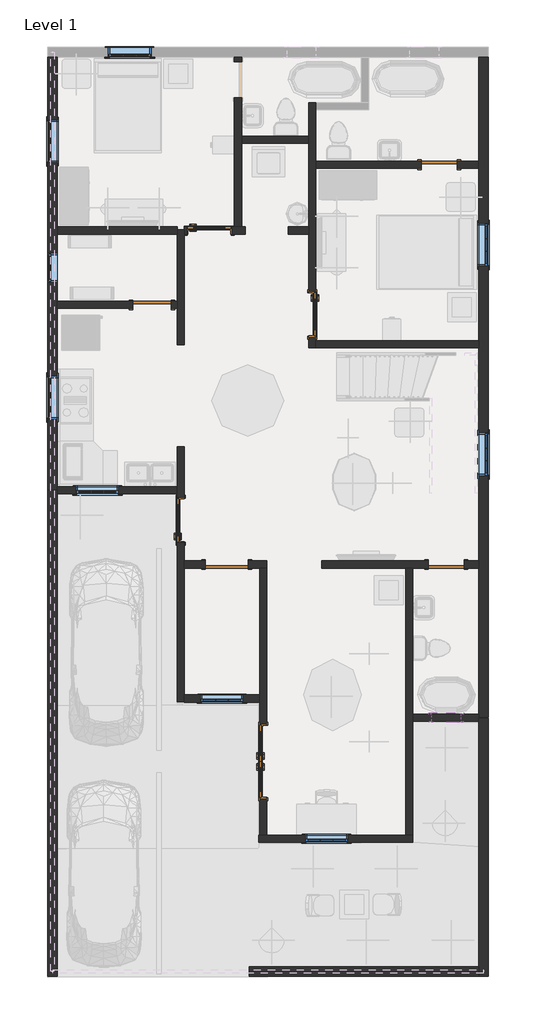
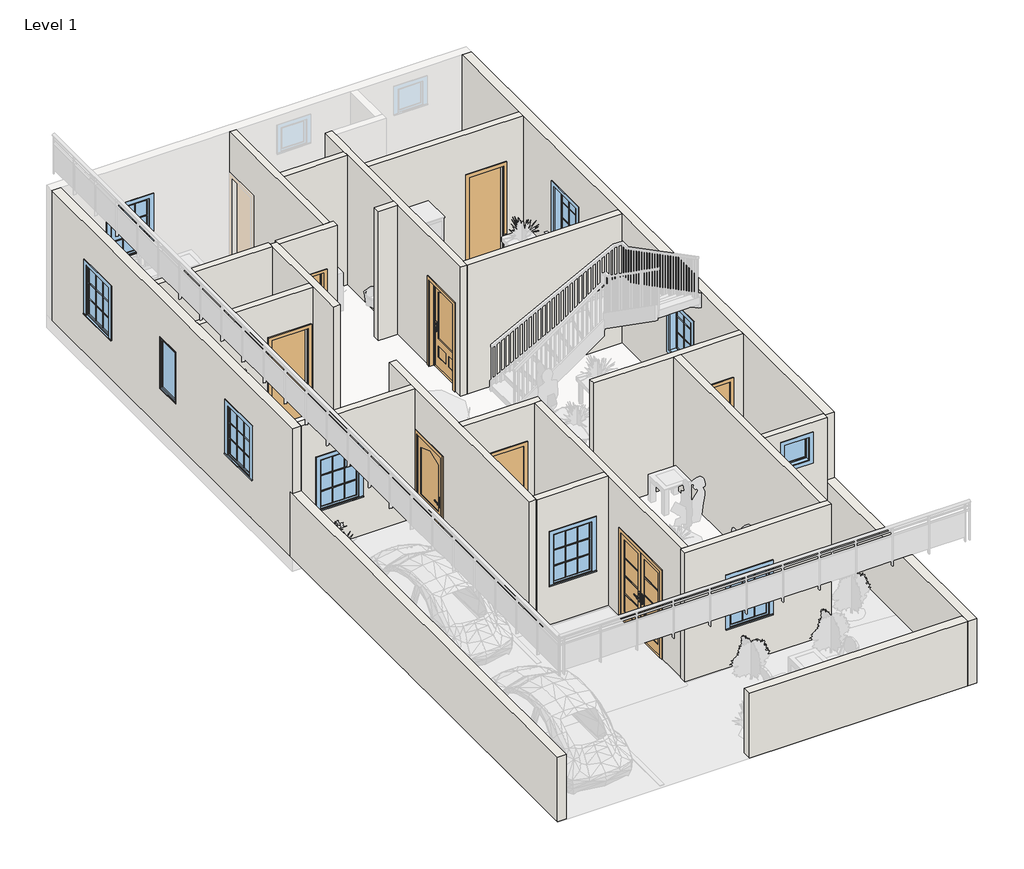
# One storey, part 1 of 4: 24 walls, 10 windows, 8 doors.
"""IFC4 building model written with IfcOpenShell, lengths in millimetres."""

from ifc_helpers import new_model, si_unit, frame, origin, origin_with_axes, place, context, project, spatial, polyline, outline, extrude, faceted_brep, transform, mapped, element, save
from components import door_5d363d20, door_94998e6c, door_255cab33, door_059fdd7e, door_377e7377, door_686f89d2, window_ce5e1bf6, window_29c06734, window_5c190c7e, window_80bd9af0, window_3d781103

model = new_model("IFC4")

# Units and contexts
model_context = context("Model", 3, world=origin())
ifc_project = project(units=[si_unit("LENGTHUNIT", "METRE", prefix="MILLI")], contexts=[model_context])

# Site, building, storey
site = spatial("IfcSite", under=ifc_project)
building = spatial("IfcBuilding", under=site)
storey = spatial("IfcBuildingStorey", under=building, Name="Level 1", Elevation=0.0)

# Doors
placement = place(None, origin())
door_shape = door_5d363d20(model_context)
element("IfcDoor", 1, ObjectType="36\" x 80\"", at=placement, inside=storey, context=model_context, shape_type="MappedRepresentation", body=[
    mapped(door_shape, transform((-8373.0976606, 9970.2021763, 0.0), x_axis=(-1.0, 0.0, 0.0), y_axis=(0.0, -1.0, 0.0), z_axis=(0.0, 0.0, 1.0))),
])
element("IfcDoor", 2, ObjectType="36\" x 80\"", at=placement, inside=storey, context=model_context, shape_type="MappedRepresentation", body=[
    mapped(door_shape, transform((-6185.5226606, 8189.0271763, 0.0), x_axis=(0.0, 1.0, 0.0), y_axis=(-1.0, 0.0, 0.0), z_axis=(0.0, 0.0, 1.0))),
])
element("IfcDoor", 3, ObjectType="36\" x 80\"", at=placement, inside=storey, context=model_context, shape_type="MappedRepresentation", body=[
    mapped(door_shape, transform((-8985.8726606, 3820.2271763, 0.0), x_axis=(0.0, -1.0, 0.0), y_axis=(1.0, 0.0, 0.0), z_axis=(0.0, 0.0, 1.0))),
])
door_2_shape = door_94998e6c(model_context)
element("IfcDoor", 4, ObjectType="Door-Exterior-Double-Full Glass-Wood_Clad : 60\" x 80\"", at=placement, inside=storey, context=model_context, shape_type="MappedRepresentation", body=[
    mapped(door_2_shape, transform((-7233.2726606, -1297.8728237, 0.0), x_axis=(0.0, 1.0, 0.0), y_axis=(-1.0, 0.0, 0.0), z_axis=(0.0, 0.0, 1.0))),
])
door_3_shape = door_255cab33(model_context)
element("IfcDoor", 5, ObjectType="Single-Flush : 30\" x 80\"", at=placement, inside=storey, context=model_context, shape_type="MappedRepresentation", body=[
    mapped(door_3_shape, transform((-3343.8976606, 2880.4271763, 0.0), x_axis=(1.0, 0.0, 0.0), y_axis=(0.0, 1.0, 0.0), z_axis=(0.0, 0.0, 1.0))),
])
door_4_shape = door_059fdd7e(model_context)
element("IfcDoor", 6, ObjectType="Single-Flush : 30\" x 80\"", at=placement, inside=storey, context=model_context, shape_type="MappedRepresentation", body=[
    mapped(door_4_shape, transform((-3496.2976606, 11364.0271763, 0.0), x_axis=(1.0, 0.0, 0.0), y_axis=(0.0, 1.0, 0.0), z_axis=(0.0, 0.0, 1.0))),
])
door_5_shape = door_377e7377(model_context)
element("IfcDoor", 7, ObjectType="Single-Flush : 32\" x 84\"", at=placement, inside=storey, context=model_context, shape_type="MappedRepresentation", body=[
    mapped(door_5_shape, transform((-9592.2976606, 8392.2271763, 0.0), x_axis=(1.0, 0.0, 0.0), y_axis=(0.0, 1.0, 0.0), z_axis=(0.0, 0.0, 1.0))),
])
door_6_shape = door_686f89d2(model_context)
element("IfcDoor", 8, ObjectType="Single-Flush : 36\" x 84\"", at=placement, inside=storey, context=model_context, shape_type="MappedRepresentation", body=[
    mapped(door_6_shape, transform((-8004.7976606, 2880.4271763, 0.0), x_axis=(1.0, 0.0, 0.0), y_axis=(0.0, 1.0, 0.0), z_axis=(0.0, 0.0, 1.0))),
])

# Walls
element("IfcWall", 9, ObjectType="Generic - 5'", at=placement, inside=storey, context=model_context, shape_type="Brep", body=[
    faceted_brep([(-11598.8976606, -5857.1728237, 0.0), (-11598.8976606, 4379.0271763, 0.0), (-11598.8976606, 4455.2271763, 0.0), (-11598.8976606, 4455.2271763, 1524.0), (-11598.8976606, -5857.1728237, 1524.0), (-11802.0976606, -5857.1728237, 0.0), (-11802.0976606, -5857.1728237, 1524.0), (-11802.0976606, 4455.2271763, 1524.0), (-11802.0976606, 4455.2271763, 0.0)], [[[0, 1, 2, 3, 4]], [[5, 6, 7, 8]], [[2, 1, 0, 5, 8]], [[3, 2, 8, 7]], [[4, 3, 7, 6]], [[0, 4, 6, 5]]]),
])
element("IfcWall", 10, ObjectType="Generic - 5'", at=placement, inside=storey, context=model_context, shape_type="Brep", body=[
    faceted_brep([(-2658.0976606, -383.4728237, 0.0), (-2658.0976606, -446.9728237, 0.0), (-2658.0976606, -5653.9728237, 0.0), (-2658.0976606, -5857.1728237, 0.0), (-2658.0976606, -5857.1728237, 1524.0), (-2658.0976606, -5653.9728237, 1524.0), (-2658.0976606, -383.4728237, 1524.0), (-2454.8976606, -383.4728237, 0.0), (-2454.8976606, -383.4728237, 1524.0), (-2454.8976606, -5857.1728237, 1524.0), (-2454.8976606, -5857.1728237, 0.0)], [[[0, 1, 2, 3, 4, 5, 6]], [[7, 8, 9, 10]], [[3, 2, 1, 0, 7, 10]], [[6, 5, 4, 9, 8]], [[0, 6, 8, 7]], [[4, 3, 10, 9]]]),
])
element("IfcWall", 11, ObjectType="Generic - 5'", at=placement, inside=storey, context=model_context, shape_type="SweptSolid", body=[
    extrude(outline(polyline([(-7522.1976606, -5653.9728237), (-2658.0976606, -5653.9728237), (-2658.0976606, -5857.1728237), (-7522.1976606, -5857.1728237), (-7522.1976606, -5653.9728237)])), origin_with_axes(), (0.0, 0.0, 1.0), 1524.0),
])
element("IfcWall", 12, ObjectType="Generic - 8\"", at=placement, inside=storey, context=model_context, shape_type="Brep", body=[
    faceted_brep([(-2658.0976606, 13650.0271763, 0.0), (-2658.0976606, 11440.2271763, 0.0), (-2658.0976606, 11287.8271763, 0.0), (-2658.0976606, 7630.2271763, 0.0), (-2658.0976606, 7477.8271763, 0.0), (-2658.0976606, 2956.6271763, 0.0), (-2658.0976606, 2804.2271763, 0.0), (-2658.0976606, -358.0728237, 0.0), (-2658.0976606, -358.0728237, 3048.0), (-2658.0976606, 2804.2271763, 3048.0), (-2658.0976606, 2956.6271763, 3048.0), (-2658.0976606, 7477.8271763, 3048.0), (-2658.0976606, 7630.2271763, 3048.0), (-2658.0976606, 11287.8271763, 3048.0), (-2658.0976606, 11440.2271763, 3048.0), (-2658.0976606, 13650.0271763, 3048.0), (-2658.0976606, 9205.0271763, 2133.6), (-2658.0976606, 9205.0271763, 914.4), (-2658.0976606, 10119.4271763, 914.4), (-2658.0976606, 10119.4271763, 2133.6), (-2658.0976606, 4760.0271763, 2133.6), (-2658.0976606, 4760.0271763, 914.4), (-2658.0976606, 5674.4271763, 914.4), (-2658.0976606, 5674.4271763, 2133.6), (-2454.8976606, 13650.0271763, 0.0), (-2454.8976606, 13650.0271763, 3048.0), (-2454.8976606, -358.0728237, 3048.0), (-2454.8976606, -358.0728237, 0.0), (-2454.8976606, 9205.0271763, 2133.6), (-2454.8976606, 10119.4271763, 2133.6), (-2454.8976606, 10119.4271763, 914.4), (-2454.8976606, 9205.0271763, 914.4), (-2454.8976606, 4760.0271763, 2133.6), (-2454.8976606, 5674.4271763, 2133.6), (-2454.8976606, 5674.4271763, 914.4), (-2454.8976606, 4760.0271763, 914.4)], [[[0, 1, 2, 3, 4, 5, 6, 7, 8, 9, 10, 11, 12, 13, 14, 15], [16, 17, 18, 19], [20, 21, 22, 23]], [[24, 25, 26, 27], [28, 29, 30, 31], [32, 33, 34, 35]], [[7, 6, 5, 4, 3, 2, 1, 0, 24, 27]], [[8, 7, 27, 26]], [[0, 15, 25, 24]], [[17, 16, 28, 31]], [[18, 17, 31, 30]], [[19, 18, 30, 29]], [[16, 19, 29, 28]], [[21, 20, 32, 35]], [[22, 21, 35, 34]], [[23, 22, 34, 33]], [[20, 23, 33, 32]], [[15, 14, 13, 12, 11, 10, 9, 8, 26, 25]]]),
])
element("IfcWall", 13, ObjectType="Generic - 8\"", at=placement, inside=storey, context=model_context, shape_type="Brep", body=[
    faceted_brep([(-11598.8976606, 4455.2271763, 0.0), (-11598.8976606, 4531.4271763, 0.0), (-11598.8976606, 8316.0271763, 0.0), (-11598.8976606, 8468.4271763, 0.0), (-11598.8976606, 9890.8271763, 0.0), (-11598.8976606, 10043.2271763, 0.0), (-11598.8976606, 13650.0271763, 0.0), (-11598.8976606, 13650.0271763, 3048.0), (-11598.8976606, 10043.2271763, 3048.0), (-11598.8976606, 9890.8271763, 3048.0), (-11598.8976606, 8468.4271763, 3048.0), (-11598.8976606, 8316.0271763, 3048.0), (-11598.8976606, 4531.4271763, 3048.0), (-11598.8976606, 4379.0271763, 3048.0), (-11598.8976606, 4379.0271763, 1524.0), (-11598.8976606, 4455.2271763, 1524.0), (-11598.8976606, 12316.5271763, 2133.6), (-11598.8976606, 12316.5271763, 914.4), (-11598.8976606, 11402.1271763, 914.4), (-11598.8976606, 11402.1271763, 2133.6), (-11598.8976606, 6880.9271763, 2133.6), (-11598.8976606, 6880.9271763, 914.4), (-11598.8976606, 5966.5271763, 914.4), (-11598.8976606, 5966.5271763, 2133.6), (-11598.8976606, 9484.4271763, 2133.6), (-11598.8976606, 9484.4271763, 914.4), (-11598.8976606, 8874.8271763, 914.4), (-11598.8976606, 8874.8271763, 2133.6), (-11802.0976606, 4455.2271763, 0.0), (-11802.0976606, 4455.2271763, 1524.0), (-11802.0976606, 4379.0271763, 1524.0), (-11802.0976606, 4379.0271763, 3048.0), (-11802.0976606, 13650.0271763, 3048.0), (-11802.0976606, 13650.0271763, 0.0), (-11802.0976606, 12316.5271763, 2133.6), (-11802.0976606, 11402.1271763, 2133.6), (-11802.0976606, 11402.1271763, 914.4), (-11802.0976606, 12316.5271763, 914.4), (-11802.0976606, 6880.9271763, 2133.6), (-11802.0976606, 5966.5271763, 2133.6), (-11802.0976606, 5966.5271763, 914.4), (-11802.0976606, 6880.9271763, 914.4), (-11802.0976606, 9484.4271763, 2133.6), (-11802.0976606, 8874.8271763, 2133.6), (-11802.0976606, 8874.8271763, 914.4), (-11802.0976606, 9484.4271763, 914.4)], [[[0, 1, 2, 3, 4, 5, 6, 7, 8, 9, 10, 11, 12, 13, 14, 15], [16, 17, 18, 19], [20, 21, 22, 23], [24, 25, 26, 27]], [[28, 29, 30, 31, 32, 33], [34, 35, 36, 37], [38, 39, 40, 41], [42, 43, 44, 45]], [[6, 5, 4, 3, 2, 1, 0, 28, 33]], [[7, 6, 33, 32]], [[16, 19, 35, 34]], [[19, 18, 36, 35]], [[18, 17, 37, 36]], [[17, 16, 34, 37]], [[20, 23, 39, 38]], [[23, 22, 40, 39]], [[22, 21, 41, 40]], [[21, 20, 38, 41]], [[24, 27, 43, 42]], [[27, 26, 44, 43]], [[26, 25, 45, 44]], [[25, 24, 42, 45]], [[0, 15, 29, 28]], [[14, 30, 29, 15]], [[14, 13, 31, 30]], [[13, 12, 11, 10, 9, 8, 7, 32, 31]]]),
])
element("IfcWall", 14, ObjectType="inner 6\"", at=placement, inside=storey, context=model_context, shape_type="Brep", body=[
    faceted_brep([(-9058.8976606, 10043.2271763, 0.0), (-11598.8976606, 10043.2271763, 0.0), (-11598.8976606, 10043.2271763, 3048.0), (-9058.8976606, 10043.2271763, 3048.0), (-9058.8976606, 9890.8271763, 0.0), (-9058.8976606, 9890.8271763, 3048.0), (-11598.8976606, 9890.8271763, 3048.0), (-11598.8976606, 9890.8271763, 0.0), (-9058.8976606, 9979.7271763, 0.0), (-9058.8976606, 9979.7271763, 3048.0)], [[[0, 1, 2, 3]], [[4, 5, 6, 7]], [[1, 0, 8, 4, 7]], [[0, 3, 9, 5, 4, 8]], [[2, 1, 7, 6]], [[3, 2, 6, 5, 9]]]),
])
element("IfcWall", 15, ObjectType="inner 6\"", at=placement, inside=storey, context=model_context, shape_type="SweptSolid", body=[
    extrude(outline(polyline([(-6264.8976606, 11821.2271763), (-7687.2976606, 11821.2271763), (-7687.2976606, 11973.6271763), (-6264.8976606, 11973.6271763), (-6264.8976606, 11821.2271763)])), origin_with_axes(), (0.0, 0.0, 1.0), 3048.0),
])
element("IfcWall", 16, ObjectType="inner 6\"", at=placement, inside=storey, context=model_context, shape_type="Brep", body=[
    faceted_brep([(-6112.4976606, 12684.8271763, 0.0), (-6112.4976606, 12684.8271763, 3048.0), (-6112.4976606, 12532.4271763, 3048.0), (-6112.4976606, 11440.2271763, 3048.0), (-6112.4976606, 11287.8271763, 3048.0), (-6112.4976606, 7630.2271763, 3048.0), (-6112.4976606, 7477.8271763, 3048.0), (-6112.4976606, 7477.8271763, 0.0), (-6112.4976606, 7630.2271763, 0.0), (-6112.4976606, 7706.4271763, 0.0), (-6112.4976606, 7706.4271763, 2057.4), (-6112.4976606, 8671.6271763, 2057.4), (-6112.4976606, 8671.6271763, 0.0), (-6112.4976606, 11287.8271763, 0.0), (-6112.4976606, 11440.2271763, 0.0), (-6112.4976606, 12532.4271763, 0.0), (-6264.8976606, 12684.8271763, 3048.0), (-6264.8976606, 12684.8271763, 0.0), (-6264.8976606, 11973.6271763, 0.0), (-6264.8976606, 11821.2271763, 0.0), (-6264.8976606, 10043.2271763, 0.0), (-6264.8976606, 9890.8271763, 0.0), (-6264.8976606, 8671.6271763, 0.0), (-6264.8976606, 8671.6271763, 2057.4), (-6264.8976606, 7706.4271763, 2057.4), (-6264.8976606, 7706.4271763, 0.0), (-6264.8976606, 7477.8271763, 0.0), (-6264.8976606, 7477.8271763, 3048.0), (-6264.8976606, 9890.8271763, 3048.0), (-6264.8976606, 10043.2271763, 3048.0), (-6264.8976606, 11821.2271763, 3048.0), (-6264.8976606, 11973.6271763, 3048.0)], [[[0, 1, 2, 3, 4, 5, 6, 7, 8, 9, 10, 11, 12, 13, 14, 15]], [[16, 17, 18, 19, 20, 21, 22, 23, 24, 25, 26, 27, 28, 29, 30, 31]], [[17, 0, 15, 14, 13, 12, 22, 21, 20, 19, 18]], [[7, 26, 25, 9, 8]], [[1, 0, 17, 16]], [[7, 6, 27, 26]], [[11, 23, 22, 12]], [[23, 11, 10, 24]], [[24, 10, 9, 25]], [[6, 5, 4, 3, 2, 1, 16, 31, 30, 29, 28, 27]]]),
])
element("IfcWall", 17, ObjectType="inner 6\"", at=placement, inside=storey, context=model_context, shape_type="SweptSolid", body=[
    extrude(outline(polyline([(-6112.4976606, 7630.2271763), (-2658.0976606, 7630.2271763), (-2658.0976606, 7477.8271763), (-6112.4976606, 7477.8271763), (-6112.4976606, 7630.2271763)])), origin_with_axes(), (0.0, 0.0, 1.0), 3048.0),
])
element("IfcWall", 18, ObjectType="inner 6\"", at=placement, inside=storey, context=model_context, shape_type="SweptSolid", body=[
    extrude(outline(polyline([(2032.0, -3115.2976606), (0.0, -3115.2976606), (0.0, -2658.0976606), (3048.0, -2658.0976606), (3048.0, -6112.4976606), (0.0, -6112.4976606), (0.0, -3877.2976606), (2032.0, -3877.2976606), (2032.0, -3115.2976606)])), frame((0.0, 11287.8271763, 0.0), z_axis=(0.0, 1.0, 0.0), x_axis=(0.0, 0.0, 1.0)), (0.0, 0.0, 1.0), 152.4),
])
element("IfcWall", 19, ObjectType="inner 6\"", at=placement, inside=storey, context=model_context, shape_type="SweptSolid", body=[
    extrude(outline(polyline([(2133.6, -9185.8976606), (0.0, -9185.8976606), (0.0, -9058.8976606), (3048.0, -9058.8976606), (3048.0, -11598.8976606), (0.0, -11598.8976606), (0.0, -9998.6976606), (2133.6, -9998.6976606), (2133.6, -9185.8976606)])), frame((0.0, 8316.0271763, 0.0), z_axis=(0.0, 1.0, 0.0), x_axis=(0.0, 0.0, 1.0)), (0.0, 0.0, 1.0), 152.4),
])
element("IfcWall", 20, ObjectType="inner 6\"", at=placement, inside=storey, context=model_context, shape_type="Brep", body=[
    faceted_brep([(-11598.8976606, 4379.0271763, 3048.0), (-11598.8976606, 4379.0271763, 1524.0), (-11598.8976606, 4379.0271763, 0.0), (-9058.8976606, 4379.0271763, 0.0), (-9058.8976606, 4379.0271763, 3048.0), (-11205.1976606, 4379.0271763, 2133.6), (-10290.7976606, 4379.0271763, 2133.6), (-10290.7976606, 4379.0271763, 914.4), (-11205.1976606, 4379.0271763, 914.4), (-11598.8976606, 4531.4271763, 0.0), (-11598.8976606, 4531.4271763, 3048.0), (-9058.8976606, 4531.4271763, 3048.0), (-9058.8976606, 4531.4271763, 0.0), (-11205.1976606, 4531.4271763, 2133.6), (-11205.1976606, 4531.4271763, 914.4), (-10290.7976606, 4531.4271763, 914.4), (-10290.7976606, 4531.4271763, 2133.6), (-11598.8976606, 4455.2271763, 0.0)], [[[0, 1, 2, 3, 4], [5, 6, 7, 8]], [[9, 10, 11, 12], [13, 14, 15, 16]], [[3, 2, 17, 9, 12]], [[4, 3, 12, 11]], [[14, 13, 5, 8]], [[15, 14, 8, 7]], [[16, 15, 7, 6]], [[13, 16, 6, 5]], [[0, 10, 9, 17, 2, 1]], [[0, 4, 11, 10]]]),
])
element("IfcWall", 21, ObjectType="inner 6\"", at=placement, inside=storey, context=model_context, shape_type="Brep", body=[
    faceted_brep([(-4055.0976606, -2859.9728237, 0.0), (-4055.0976606, -446.9728237, 0.0), (-4055.0976606, -294.5728237, 0.0), (-4055.0976606, 2804.2271763, 0.0), (-4055.0976606, 2804.2271763, 3048.0), (-4055.0976606, -294.5728237, 3048.0), (-4055.0976606, -446.9728237, 3048.0), (-4055.0976606, -2859.9728237, 3048.0), (-4207.4976606, -2859.9728237, 0.0), (-4207.4976606, -2859.9728237, 3048.0), (-4207.4976606, 2804.2271763, 3048.0), (-4207.4976606, 2804.2271763, 0.0)], [[[0, 1, 2, 3, 4, 5, 6, 7]], [[8, 9, 10, 11]], [[3, 2, 1, 0, 8, 11]], [[0, 7, 9, 8]], [[4, 3, 11, 10]], [[7, 6, 5, 4, 10, 9]]]),
])
element("IfcWall", 22, ObjectType="inner 6\"", at=placement, inside=storey, context=model_context, shape_type="Brep", body=[
    faceted_brep([(-4055.0976606, -446.9728237, 0.0), (-2658.0976606, -446.9728237, 0.0), (-2658.0976606, -446.9728237, 3048.0), (-4055.0976606, -446.9728237, 3048.0), (-3039.0976606, -446.9728237, 2768.6), (-3039.0976606, -446.9728237, 2159.0), (-3648.6976606, -446.9728237, 2159.0), (-3648.6976606, -446.9728237, 2768.6), (-4055.0976606, -294.5728237, 0.0), (-4055.0976606, -294.5728237, 3048.0), (-2658.0976606, -294.5728237, 3048.0), (-2658.0976606, -294.5728237, 0.0), (-3039.0976606, -294.5728237, 2768.6), (-3648.6976606, -294.5728237, 2768.6), (-3648.6976606, -294.5728237, 2159.0), (-3039.0976606, -294.5728237, 2159.0), (-2658.0976606, -383.4728237, 0.0)], [[[0, 1, 2, 3], [4, 5, 6, 7]], [[8, 9, 10, 11], [12, 13, 14, 15]], [[1, 0, 8, 11, 16]], [[0, 3, 9, 8]], [[2, 1, 16, 11, 10]], [[5, 4, 12, 15]], [[6, 5, 15, 14]], [[7, 6, 14, 13]], [[4, 7, 13, 12]], [[3, 2, 10, 9]]]),
])
element("IfcWall", 23, ObjectType="inner 6\"", at=placement, inside=storey, context=model_context, shape_type="Brep", body=[
    faceted_brep([(-2962.8976606, 2804.2271763, 2032.0), (-2962.8976606, 2804.2271763, 0.0), (-2658.0976606, 2804.2271763, 0.0), (-2658.0976606, 2804.2271763, 3048.0), (-4055.0976606, 2804.2271763, 3048.0), (-4207.4976606, 2804.2271763, 3048.0), (-5985.4976606, 2804.2271763, 3048.0), (-5985.4976606, 2804.2271763, 0.0), (-4207.4976606, 2804.2271763, 0.0), (-4055.0976606, 2804.2271763, 0.0), (-3724.8976606, 2804.2271763, 0.0), (-3724.8976606, 2804.2271763, 2032.0), (-2658.0976606, 2956.6271763, 0.0), (-2962.8976606, 2956.6271763, 0.0), (-2962.8976606, 2956.6271763, 2032.0), (-3724.8976606, 2956.6271763, 2032.0), (-3724.8976606, 2956.6271763, 0.0), (-5985.4976606, 2956.6271763, 0.0), (-5985.4976606, 2956.6271763, 3048.0), (-2658.0976606, 2956.6271763, 3048.0)], [[[0, 1, 2, 3, 4, 5, 6, 7, 8, 9, 10, 11]], [[12, 13, 14, 15, 16, 17, 18, 19]], [[2, 1, 13, 12]], [[10, 9, 8, 7, 17, 16]], [[7, 6, 18, 17]], [[3, 2, 12, 19]], [[14, 13, 1, 0]], [[15, 14, 0, 11]], [[16, 15, 11, 10]], [[6, 5, 4, 3, 19, 18]]]),
])
element("IfcWall", 24, ObjectType="inner 6\"", at=placement, inside=storey, context=model_context, shape_type="Brep", body=[
    faceted_brep([(-7153.8976606, 2956.6271763, 0.0), (-7547.5976606, 2956.6271763, 0.0), (-7547.5976606, 2956.6271763, 2133.6), (-8461.9976606, 2956.6271763, 2133.6), (-8461.9976606, 2956.6271763, 0.0), (-8906.4976606, 2956.6271763, 0.0), (-8906.4976606, 2956.6271763, 3048.0), (-7153.8976606, 2956.6271763, 3048.0), (-7547.5976606, 2804.2271763, 2133.6), (-7547.5976606, 2804.2271763, 0.0), (-7306.2976606, 2804.2271763, 0.0), (-7153.8976606, 2804.2271763, 0.0), (-7153.8976606, 2804.2271763, 3048.0), (-7306.2976606, 2804.2271763, 3048.0), (-8906.4976606, 2804.2271763, 3048.0), (-8906.4976606, 2804.2271763, 0.0), (-8461.9976606, 2804.2271763, 0.0), (-8461.9976606, 2804.2271763, 2133.6)], [[[0, 1, 2, 3, 4, 5, 6, 7]], [[8, 9, 10, 11, 12, 13, 14, 15, 16, 17]], [[16, 15, 5, 4]], [[11, 10, 9, 1, 0]], [[0, 7, 12, 11]], [[6, 5, 15, 14]], [[2, 1, 9, 8]], [[3, 2, 8, 17]], [[4, 3, 17, 16]], [[7, 6, 14, 13, 12]]]),
])
element("IfcWall", 25, ObjectType="inner 6\"", at=placement, inside=storey, context=model_context, shape_type="Brep", body=[
    faceted_brep([(-7306.2976606, -2859.9728237, 0.0), (-7306.2976606, -2859.9728237, 3048.0), (-7306.2976606, -40.5728237, 3048.0), (-7306.2976606, 111.8271763, 3048.0), (-7306.2976606, 2804.2271763, 3048.0), (-7306.2976606, 2804.2271763, 0.0), (-7306.2976606, 111.8271763, 0.0), (-7306.2976606, -40.5728237, 0.0), (-7306.2976606, -510.4728237, 0.0), (-7306.2976606, -510.4728237, 2057.4), (-7306.2976606, -2085.2728237, 2057.4), (-7306.2976606, -2085.2728237, 0.0), (-7153.8976606, -2859.9728237, 3048.0), (-7153.8976606, -2859.9728237, 0.0), (-7153.8976606, -2085.2728237, 0.0), (-7153.8976606, -2085.2728237, 2057.4), (-7153.8976606, -510.4728237, 2057.4), (-7153.8976606, -510.4728237, 0.0), (-7153.8976606, 2804.2271763, 0.0), (-7153.8976606, 2804.2271763, 3048.0)], [[[0, 1, 2, 3, 4, 5, 6, 7, 8, 9, 10, 11]], [[12, 13, 14, 15, 16, 17, 18, 19]], [[13, 0, 11, 14]], [[5, 18, 17, 8, 7, 6]], [[1, 0, 13, 12]], [[5, 4, 19, 18]], [[16, 9, 8, 17]], [[9, 16, 15, 10]], [[10, 15, 14, 11]], [[4, 3, 2, 1, 12, 19]]]),
])
element("IfcWall", 26, ObjectType="inner 6\"", at=placement, inside=storey, context=model_context, shape_type="Brep", body=[
    faceted_brep([(-9058.8976606, 9979.7271763, 0.0), (-9058.8976606, 9890.8271763, 0.0), (-9058.8976606, 8468.4271763, 0.0), (-9058.8976606, 8316.0271763, 0.0), (-9058.8976606, 7541.3271763, 0.0), (-9058.8976606, 7541.3271763, 3048.0), (-9058.8976606, 8316.0271763, 3048.0), (-9058.8976606, 8468.4271763, 3048.0), (-9058.8976606, 9890.8271763, 3048.0), (-9058.8976606, 9979.7271763, 3048.0), (-8906.4976606, 9979.7271763, 0.0), (-8906.4976606, 9979.7271763, 3048.0), (-8906.4976606, 9890.8271763, 3048.0), (-8906.4976606, 7541.3271763, 3048.0), (-8906.4976606, 7541.3271763, 0.0), (-8906.4976606, 9890.8271763, 0.0)], [[[0, 1, 2, 3, 4, 5, 6, 7, 8, 9]], [[10, 11, 12, 13, 14, 15]], [[4, 3, 2, 1, 0, 10, 15, 14]], [[5, 4, 14, 13]], [[0, 9, 11, 10]], [[9, 8, 7, 6, 5, 13, 12, 11]]]),
])
element("IfcWall", 27, ObjectType="inner 6\"", at=placement, inside=storey, context=model_context, shape_type="Brep", body=[
    faceted_brep([(-7839.6976606, 13650.0271763, 0.0), (-7839.6976606, 13548.4271763, 0.0), (-7839.6976606, 13548.4271763, 2032.0), (-7839.6976606, 12786.4271763, 2032.0), (-7839.6976606, 12786.4271763, 0.0), (-7839.6976606, 10043.2271763, 0.0), (-7839.6976606, 10043.2271763, 3048.0), (-7839.6976606, 13650.0271763, 3048.0), (-7687.2976606, 13548.4271763, 2032.0), (-7687.2976606, 13548.4271763, 0.0), (-7687.2976606, 13650.0271763, 0.0), (-7687.2976606, 13650.0271763, 3048.0), (-7687.2976606, 11973.6271763, 3048.0), (-7687.2976606, 11821.2271763, 3048.0), (-7687.2976606, 10043.2271763, 3048.0), (-7687.2976606, 10043.2271763, 0.0), (-7687.2976606, 11821.2271763, 0.0), (-7687.2976606, 11973.6271763, 0.0), (-7687.2976606, 12786.4271763, 0.0), (-7687.2976606, 12786.4271763, 2032.0)], [[[0, 1, 2, 3, 4, 5, 6, 7]], [[8, 9, 10, 11, 12, 13, 14, 15, 16, 17, 18, 19]], [[10, 9, 1, 0]], [[18, 17, 16, 15, 5, 4]], [[0, 7, 11, 10]], [[6, 5, 15, 14]], [[2, 1, 9, 8]], [[3, 2, 8, 19]], [[4, 3, 19, 18]], [[7, 6, 14, 13, 12, 11]]]),
])
element("IfcWall", 28, ObjectType="inner 6\"", at=placement, inside=storey, context=model_context, shape_type="Brep", body=[
    faceted_brep([(-7611.0976606, 9890.8271763, 0.0), (-7611.0976606, 9890.8271763, 3048.0), (-8906.4976606, 9890.8271763, 3048.0), (-8906.4976606, 9890.8271763, 0.0), (-8855.6976606, 9890.8271763, 0.0), (-8855.6976606, 9890.8271763, 2057.4), (-7890.4976606, 9890.8271763, 2057.4), (-7890.4976606, 9890.8271763, 0.0), (-7611.0976606, 10043.2271763, 3048.0), (-7611.0976606, 10043.2271763, 0.0), (-7687.2976606, 10043.2271763, 0.0), (-7839.6976606, 10043.2271763, 0.0), (-7890.4976606, 10043.2271763, 0.0), (-7890.4976606, 10043.2271763, 2057.4), (-8855.6976606, 10043.2271763, 2057.4), (-8855.6976606, 10043.2271763, 0.0), (-8906.4976606, 10043.2271763, 0.0), (-8906.4976606, 10043.2271763, 3048.0), (-7839.6976606, 10043.2271763, 3048.0), (-7687.2976606, 10043.2271763, 3048.0), (-8906.4976606, 9979.7271763, 0.0), (-8906.4976606, 9979.7271763, 3048.0)], [[[0, 1, 2, 3, 4, 5, 6, 7]], [[8, 9, 10, 11, 12, 13, 14, 15, 16, 17, 18, 19]], [[9, 0, 7, 12, 11, 10]], [[3, 20, 16, 15, 4]], [[1, 0, 9, 8]], [[3, 2, 21, 17, 16, 20]], [[5, 14, 13, 6]], [[6, 13, 12, 7]], [[14, 5, 4, 15]], [[2, 1, 8, 19, 18, 17, 21]]]),
])
element("IfcWall", 29, ObjectType="inner 6\"", at=placement, inside=storey, context=model_context, shape_type="SweptSolid", body=[
    extrude(outline(polyline([(-6264.8976606, 9890.8271763), (-6696.6976606, 9890.8271763), (-6696.6976606, 10043.2271763), (-6264.8976606, 10043.2271763), (-6264.8976606, 9890.8271763)])), origin_with_axes(), (0.0, 0.0, 1.0), 3048.0),
])
element("IfcWall", 30, ObjectType="inner 6\"", at=placement, inside=storey, context=model_context, shape_type="Brep", body=[
    faceted_brep([(-9058.8976606, -27.8728237, 0.0), (-9058.8976606, -27.8728237, 3048.0), (-9058.8976606, 4379.0271763, 3048.0), (-9058.8976606, 4531.4271763, 3048.0), (-9058.8976606, 5382.3271763, 3048.0), (-9058.8976606, 5382.3271763, 0.0), (-9058.8976606, 4531.4271763, 0.0), (-9058.8976606, 4379.0271763, 0.0), (-9058.8976606, 4302.8271763, 0.0), (-9058.8976606, 4302.8271763, 2057.4), (-9058.8976606, 3337.6271763, 2057.4), (-9058.8976606, 3337.6271763, 0.0), (-8906.4976606, -27.8728237, 3048.0), (-8906.4976606, -27.8728237, 0.0), (-8906.4976606, 111.8271763, 0.0), (-8906.4976606, 2804.2271763, 0.0), (-8906.4976606, 2956.6271763, 0.0), (-8906.4976606, 3337.6271763, 0.0), (-8906.4976606, 3337.6271763, 2057.4), (-8906.4976606, 4302.8271763, 2057.4), (-8906.4976606, 4302.8271763, 0.0), (-8906.4976606, 5382.3271763, 0.0), (-8906.4976606, 5382.3271763, 3048.0), (-8906.4976606, 2956.6271763, 3048.0), (-8906.4976606, 2804.2271763, 3048.0), (-8906.4976606, 111.8271763, 3048.0)], [[[0, 1, 2, 3, 4, 5, 6, 7, 8, 9, 10, 11]], [[12, 13, 14, 15, 16, 17, 18, 19, 20, 21, 22, 23, 24, 25]], [[13, 0, 11, 17, 16, 15, 14]], [[5, 21, 20, 8, 7, 6]], [[1, 0, 13, 12]], [[5, 4, 22, 21]], [[10, 18, 17, 11]], [[18, 10, 9, 19]], [[19, 9, 8, 20]], [[4, 3, 2, 1, 12, 25, 24, 23, 22]]]),
])
element("IfcWall", 31, ObjectType="inner 6\"", at=placement, inside=storey, context=model_context, shape_type="Brep", body=[
    faceted_brep([(-8906.4976606, -40.5728237, 0.0), (-7306.2976606, -40.5728237, 0.0), (-7306.2976606, -40.5728237, 3048.0), (-8906.4976606, -40.5728237, 3048.0), (-8563.5976606, -40.5728237, 2133.6), (-7649.1976606, -40.5728237, 2133.6), (-7649.1976606, -40.5728237, 914.4), (-8563.5976606, -40.5728237, 914.4), (-8906.4976606, 111.8271763, 0.0), (-8906.4976606, 111.8271763, 3048.0), (-7306.2976606, 111.8271763, 3048.0), (-7306.2976606, 111.8271763, 0.0), (-8563.5976606, 111.8271763, 2133.6), (-8563.5976606, 111.8271763, 914.4), (-7649.1976606, 111.8271763, 914.4), (-7649.1976606, 111.8271763, 2133.6), (-8906.4976606, -27.8728237, 0.0), (-8906.4976606, -27.8728237, 3048.0)], [[[0, 1, 2, 3], [4, 5, 6, 7]], [[8, 9, 10, 11], [12, 13, 14, 15]], [[1, 0, 16, 8, 11]], [[2, 1, 11, 10]], [[13, 12, 4, 7]], [[14, 13, 7, 6]], [[15, 14, 6, 5]], [[12, 15, 5, 4]], [[0, 3, 17, 9, 8, 16]], [[3, 2, 10, 9, 17]]]),
])
element("IfcWall", 32, ObjectType="inner 6\"", at=placement, inside=storey, context=model_context, shape_type="Brep", body=[
    faceted_brep([(-7318.9976606, -3012.3728237, 0.0), (-4055.0976606, -3012.3728237, 0.0), (-4055.0976606, -3012.3728237, 3048.0), (-7318.9976606, -3012.3728237, 3048.0), (-6341.0976606, -3012.3728237, 2133.6), (-5426.6976606, -3012.3728237, 2133.6), (-5426.6976606, -3012.3728237, 914.4), (-6341.0976606, -3012.3728237, 914.4), (-7318.9976606, -2859.9728237, 0.0), (-7318.9976606, -2859.9728237, 3048.0), (-7306.2976606, -2859.9728237, 3048.0), (-7153.8976606, -2859.9728237, 3048.0), (-4207.4976606, -2859.9728237, 3048.0), (-4055.0976606, -2859.9728237, 3048.0), (-4055.0976606, -2859.9728237, 0.0), (-4207.4976606, -2859.9728237, 0.0), (-7153.8976606, -2859.9728237, 0.0), (-7306.2976606, -2859.9728237, 0.0), (-6341.0976606, -2859.9728237, 2133.6), (-6341.0976606, -2859.9728237, 914.4), (-5426.6976606, -2859.9728237, 914.4), (-5426.6976606, -2859.9728237, 2133.6)], [[[0, 1, 2, 3], [4, 5, 6, 7]], [[8, 9, 10, 11, 12, 13, 14, 15, 16, 17], [18, 19, 20, 21]], [[1, 0, 8, 17, 16, 15, 14]], [[0, 3, 9, 8]], [[2, 1, 14, 13]], [[19, 18, 4, 7]], [[20, 19, 7, 6]], [[21, 20, 6, 5]], [[18, 21, 5, 4]], [[3, 2, 13, 12, 11, 10, 9]]]),
])

# Windows
window_shape = window_ce5e1bf6(model_context)
element("IfcWindow", 33, ObjectType="Casement 3x3 with Trim : 36\" x 48\"", at=placement, inside=storey, context=model_context, shape_type="MappedRepresentation", body=[
    mapped(window_shape, transform((-10062.1976606, 13751.6271763, 0.0), x_axis=(1.0, 0.0, 0.0), y_axis=(0.0, 1.0, 0.0), z_axis=(0.0, 0.0, 1.0))),
])
window_2_shape = window_29c06734(model_context)
element("IfcWindow", 34, ObjectType="Casement 3x3 with Trim : 36\" x 48\"", at=placement, inside=storey, context=model_context, shape_type="MappedRepresentation", body=[
    mapped(window_2_shape, transform((-11700.4976606, 11859.3271763, 0.0), x_axis=(0.0, 1.0, 0.0), y_axis=(-1.0, 0.0, 0.0), z_axis=(0.0, 0.0, 1.0))),
])
element("IfcWindow", 35, ObjectType="Casement 3x3 with Trim : 36\" x 48\"", at=placement, inside=storey, context=model_context, shape_type="MappedRepresentation", body=[
    mapped(window_2_shape, transform((-11700.4976606, 6423.7271763, 0.0), x_axis=(0.0, 1.0, 0.0), y_axis=(-1.0, 0.0, 0.0), z_axis=(0.0, 0.0, 1.0))),
])
element("IfcWindow", 36, ObjectType="Casement 3x3 with Trim : 36\" x 48\"", at=placement, inside=storey, context=model_context, shape_type="MappedRepresentation", body=[
    mapped(window_2_shape, transform((-2556.4976606, 9662.2271763, 0.0), x_axis=(0.0, -1.0, 0.0), y_axis=(1.0, 0.0, 0.0), z_axis=(0.0, 0.0, 1.0))),
])
element("IfcWindow", 37, ObjectType="Casement 3x3 with Trim : 36\" x 48\"", at=placement, inside=storey, context=model_context, shape_type="MappedRepresentation", body=[
    mapped(window_2_shape, transform((-2556.4976606, 5217.2271763, 0.0), x_axis=(0.0, -1.0, 0.0), y_axis=(1.0, 0.0, 0.0), z_axis=(0.0, 0.0, 1.0))),
])
window_3_shape = window_5c190c7e(model_context)
element("IfcWindow", 38, ObjectType="Casement 3x3 with Trim : 36\" x 48\"", at=placement, inside=storey, context=model_context, shape_type="MappedRepresentation", body=[
    mapped(window_3_shape, transform((-10747.9976606, 4455.2271763, 0.0), x_axis=(-1.0, 0.0, 0.0), y_axis=(0.0, -1.0, 0.0), z_axis=(0.0, 0.0, 1.0))),
])
element("IfcWindow", 39, ObjectType="Casement 3x3 with Trim : 36\" x 48\"", at=placement, inside=storey, context=model_context, shape_type="MappedRepresentation", body=[
    mapped(window_3_shape, transform((-5883.8976606, -2936.1728237, 0.0), x_axis=(-1.0, 0.0, 0.0), y_axis=(0.0, -1.0, 0.0), z_axis=(0.0, 0.0, 1.0))),
])
element("IfcWindow", 40, ObjectType="Casement 3x3 with Trim : 36\" x 48\"", at=placement, inside=storey, context=model_context, shape_type="MappedRepresentation", body=[
    mapped(window_3_shape, transform((-8106.3976606, 35.6271763, 0.0), x_axis=(-1.0, 0.0, 0.0), y_axis=(0.0, -1.0, 0.0), z_axis=(0.0, 0.0, 1.0))),
])
window_4_shape = window_80bd9af0(model_context)
element("IfcWindow", 41, ObjectType="Fixed : 24\" x 48\"", at=placement, inside=storey, context=model_context, shape_type="MappedRepresentation", body=[
    mapped(window_4_shape, transform((-11700.4976606, 9217.7271763, 0.0), x_axis=(0.0, 1.0, 0.0), y_axis=(-1.0, 0.0, 0.0), z_axis=(0.0, 0.0, 1.0))),
])
window_5_shape = window_3d781103(model_context)
element("IfcWindow", 42, ObjectType="Transom with Trim : 24\" x 24\"", at=placement, inside=storey, context=model_context, shape_type="MappedRepresentation", body=[
    mapped(window_5_shape, transform((-3305.7976606, -370.7728237, 0.0), x_axis=(1.0, 0.0, 0.0), y_axis=(0.0, 1.0, 0.0), z_axis=(0.0, 0.0, 1.0))),
])

save(model, "model.ifc")

# Revit data of these elements
# Type "36\" x 80\""
#   Type Mark = "8"
#   Assembly Code = "B2030100"
#   Analytic Construction = "French door, wood frame with single glass"
#   Threshold Offset [instance default] = 0' - 0 1/2"
#   Thickness = 0' - 1 3/8"
#   Thermal Resistance (R) = 1.0696 (h·ft²·°F)/BTU
#   Swing Angle [instance default] = 90.00°
#   Stiles = 0' - 4 3/4"
#   Rough Width = 3' - 2"
#   Rough Height = 6' - 9"
#   Radius = 1' - 8.05625"
#   Lock Rail = 0' - 7 1/8"
#   Height = 6' - 8"
#   Width = 3' - 0"
#   Heat Transfer Coefficient (U) = 0.9350 BTU/(h·ft²·°F)
#   Door Offset [instance default] = 0' - 0"
#   Bottom Rail = 0' - 9 1/2"
#   Threshold [instance default] = yes
#   Function = 1
#   Exterior Trim [instance default] = yes
#   Trim Material = Cherry
#   Threshold Material = Cherry
#   Panel Material = Cherry
#   Glazing = Glass
#   Frame Material = Cherry
#   Door Handle Material = Aluminum
#   Visual Light Transmittance = 0
#   Solar Heat Gain Coefficient = 0
#   Wall Closure = (empty or 0)
#   Construction Type = (empty or 0)
# Type "Door-Exterior-Double-Full Glass-Wood_Clad : 60\" x 80\""
#   Type Mark = "9"
#   Assembly Code = "B2030100"
#   Analytic Construction = "French door, wood frame with double glass"
#   Top Rail = 0' - 4 11/16"
#   Threshold Offset [instance default] = 0' - 0 1/2"
#   Thickness = 0' - 1 3/8"
#   Thermal Resistance (R) = 1.9158 (h·ft²·°F)/BTU
#   Swing Angle [instance default] = 90.00°
#   Stiles = 0' - 4 3/4"
#   Rough Width = 5' - 2"
#   Rough Height = 6' - 9"
#   Panel Width = 2' - 6"
#   Door Offset [instance default] = 0' - 0"
#   Height = 6' - 8"
#   Width = 5' - 0"
#   Heat Transfer Coefficient (U) = 0.5220 BTU/(h·ft²·°F)
#   Bottom Rail = 0' - 9 1/8"
#   Exterior Trim [instance default] = yes
#   Threshold [instance default] = yes
#   Show Grill [instance default] = yes
#   Function = 1
#   Trim Material = Cherry
#   Threshold Material = Cherry
#   Panel Material = Cherry
#   Glazing = Glass
#   Frame Material = Cherry
#   Door Handle Material = Aluminum
#   Visual Light Transmittance = 0
#   Solar Heat Gain Coefficient = 0
#   Wall Closure = (empty or 0)
#   Construction Type = (empty or 0)
# Type "Single-Flush : 30\" x 80\""
#   Type Mark = "5"
#   Construction Type Id = "MDOOR"
#   Assembly Code = "C1020"
#   Analytic Construction = "Metal"
#   Thickness = 0' - 2"
#   Heat Transfer Coefficient (U) = 0.651978 BTU/(h·ft²·°F)
#   Height = 6' - 8"
#   Trim Projection Ext = 0' - 1"
#   Trim Projection Int = 0' - 1"
#   Trim Width = 0' - 3"
#   Width = 2' - 6"
#   Define Thermal Properties by = 1
#   Door Material = Door - Panel
#   Frame Material = Door - Frame
#   Visual Light Transmittance = 0
#   Solar Heat Gain Coefficient = 0
#   Function = (empty or 0)
#   Wall Closure = (empty or 0)
# Type "Single-Flush : 32\" x 84\""
#   Type Mark = "3"
#   Construction Type Id = "MDOOR"
#   Assembly Code = "C1020"
#   Analytic Construction = "Metal"
#   Thickness = 0' - 2"
#   Heat Transfer Coefficient (U) = 0.651978 BTU/(h·ft²·°F)
#   Height = 7' - 0"
#   Trim Projection Ext = 0' - 1"
#   Trim Projection Int = 0' - 1"
#   Trim Width = 0' - 3"
#   Width = 2' - 8"
#   Define Thermal Properties by = 1
#   Door Material = Door - Panel
#   Frame Material = Door - Frame
#   Visual Light Transmittance = 0
#   Solar Heat Gain Coefficient = 0
#   Function = (empty or 0)
#   Wall Closure = (empty or 0)
# Type "Single-Flush : 36\" x 84\""
#   Type Mark = "1"
#   Construction Type Id = "MDOOR"
#   Assembly Code = "C1020"
#   Analytic Construction = "Metal"
#   Thickness = 0' - 2"
#   Heat Transfer Coefficient (U) = 0.651978 BTU/(h·ft²·°F)
#   Height = 7' - 0"
#   Trim Projection Ext = 0' - 1"
#   Trim Projection Int = 0' - 1"
#   Trim Width = 0' - 3"
#   Width = 3' - 0"
#   Define Thermal Properties by = 1
#   Door Material = Door - Panel
#   Frame Material = Door - Frame
#   Visual Light Transmittance = 0
#   Solar Heat Gain Coefficient = 0
#   Function = (empty or 0)
#   Wall Closure = (empty or 0)
# Type "Generic - 5'"
#   Assembly Code = "B2010"
#   Layers, outside or top first: 0' - 8" "Birch" (function 1)
# Type "Generic - 8\""
#   Assembly Code = "B2010"
#   Layers, outside or top first: 0' - 8" "Brick, Common" (function 1)
# Type "inner 6\""
#   Assembly Code = "B2010"
#   Layers, outside or top first: 0' - 6" "Brick, Common" (function 1)
# Type "Casement 3x3 with Trim : 36\" x 48\""
#   Type Mark = "10"
#   Construction Type Id = "GSP4R"
#   Assembly Code = "B2020100"
#   Analytic Construction = "1/8 in Pilkington single glazing"
#   Visual Light Transmittance = 0.9
#   Solar Heat Gain Coefficient = 0.78
#   Heat Transfer Coefficient (U) = 0.6496 BTU/(h·ft²·°F)
#   Height = 4' - 0"
#   Default Sill Height = 3' - 0"
#   Trim Projection - Ext. = 0' - 0 1/2"
#   Trim Projection - Int. = 0' - 0 3/4"
#   Trim Width - Exterior = 0' - 3 1/2"
#   Trim Width - Interior = 0' - 3 1/2"
#   Width = 3' - 0"
#   Window Inset = 0' - 0 3/4"
#   Define Thermal Properties by = 1
#   Glass Pane Material = Glass
#   Sash Material = Sash
#   Trim Exterior Material = Trim
#   Trim Interior Material = Trim
#   Wall Closure = (empty or 0)
# Type "Fixed : 24\" x 48\""
#   Type Mark = "2"
#   Construction Type Id = "GSP4R"
#   Assembly Code = "B2020100"
#   Analytic Construction = "1/8 in Pilkington single glazing"
#   Visual Light Transmittance = 0.9
#   Solar Heat Gain Coefficient = 0.78
#   Heat Transfer Coefficient (U) = 0.6496 BTU/(h·ft²·°F)
#   Height = 4' - 0"
#   Default Sill Height = 3' - 0"
#   Width = 2' - 0"
#   Window Inset = 0' - 0 3/4"
#   Define Thermal Properties by = 1
#   Glass Pane Material = Glass
#   Sash Material = Sash
#   Wall Closure = (empty or 0)
# Type "Transom with Trim : 24\" x 24\""
#   Type Mark = "13"
#   Construction Type Id = "GSP4R"
#   Assembly Code = "B2020100"
#   Analytic Construction = "1/8 in Pilkington single glazing"
#   Visual Light Transmittance = 0.9
#   Solar Heat Gain Coefficient = 0.78
#   Heat Transfer Coefficient (U) = 0.6496 BTU/(h·ft²·°F)
#   Height = 2' - 0"
#   Default Sill Height = 7' - 1"
#   Trim Projection - Ext. = 0' - 0 1/2"
#   Trim Projection - Int. = 0' - 0 3/4"
#   Trim Width - Exterior = 0' - 3 1/2"
#   Trim Width - Interior = 0' - 3 1/2"
#   Width = 2' - 0"
#   Window Inset = 0' - 0 3/4"
#   Define Thermal Properties by = 1
#   Glass Pane Material = Glass
#   Sash Material = Sash
#   Trim Exterior Material = Trim
#   Trim Interior Material = Trim
#   Wall Closure = (empty or 0)
# Elements 1, 2, 3 (IfcDoor, "36\" x 80\"")
#   Threshold Offset = 0' - 0 1/2"
#   Swing Angle = 90.00°
#   Door Offset = 0' - 0"
#   Threshold = yes
#   Exterior Trim = yes
#   Phase Created = New Construction
#   Materials on its faces: "Cherry", "Aluminum", "Glass"
# Element 4 (IfcDoor, "Door-Exterior-Double-Full Glass-Wood_Clad : 60\" x 80\"")
#   Threshold Offset = 0' - 0 1/2"
#   Swing Angle = 90.00°
#   Door Offset = 0' - 0"
#   Threshold = yes
#   Show Grill = yes
#   Exterior Trim = yes
#   Phase Created = New Construction
#   Materials on its faces: "Cherry", "Aluminum", "Glass"
# Elements 5, 6 (IfcDoor, "Single-Flush : 30\" x 80\"")
#   Phase Created = New Construction
#   Materials on its faces: "Door - Frame", "Door - Panel"
# Element 7 (IfcDoor, "Single-Flush : 32\" x 84\"")
#   Phase Created = New Construction
#   Materials on its faces: "Door - Frame", "Door - Panel"
# Element 8 (IfcDoor, "Single-Flush : 36\" x 84\"")
#   Phase Created = New Construction
#   Materials on its faces: "Door - Frame", "Door - Panel"
# Elements 9, 10, 11 (IfcWall, "Generic - 5'")
#   Top Offset = 0' - 0"
#   Base Offset = 0' - 0"
#   Unconnected Height = 5' - 0"
#   wall height = 5' - 0"
#   Phase Created = New Construction
#   Base Constraint = Level 1
#   Materials on its faces: "Birch"
# Elements 12, 13 (IfcWall, "Generic - 8\"")
#   Top Offset = 0' - 0"
#   Base Offset = 0' - 0"
#   Unconnected Height = 10' - 0"
#   wall height = 10' - 0"
#   Phase Created = New Construction
#   Base Constraint = Level 1
#   Materials on its faces: "Brick, Common"
# Elements 14, 15, 16, 17, 18, 19, 20, 21, 22, 23, 24, 25, 26, 27, 28, 29, 30, 31, 32 (IfcWall, "inner 6\"")
#   Top Offset = 0' - 0"
#   Base Offset = 0' - 0"
#   Unconnected Height = 10' - 0"
#   wall height = 10' - 0"
#   Phase Created = New Construction
#   Base Constraint = Level 1
#   Materials on its faces: "Brick, Common"
# Element 33 (IfcWindow, "Casement 3x3 with Trim : 36\" x 48\"")
#   Mark = "1"
#   Phase Created = New Construction
#   Materials on its faces: "Sash", "Glass", "Trim"
# Element 34 (IfcWindow, "Casement 3x3 with Trim : 36\" x 48\"")
#   Mark = "2"
#   Phase Created = New Construction
#   Materials on its faces: "Sash", "Glass", "Trim"
# Element 35 (IfcWindow, "Casement 3x3 with Trim : 36\" x 48\"")
#   Mark = "3"
#   Phase Created = New Construction
#   Materials on its faces: "Sash", "Glass", "Trim"
# Element 36 (IfcWindow, "Casement 3x3 with Trim : 36\" x 48\"")
#   Mark = "5"
#   Phase Created = New Construction
#   Materials on its faces: "Sash", "Glass", "Trim"
# Element 37 (IfcWindow, "Casement 3x3 with Trim : 36\" x 48\"")
#   Mark = "8"
#   Phase Created = New Construction
#   Materials on its faces: "Sash", "Glass", "Trim"
# Element 38 (IfcWindow, "Casement 3x3 with Trim : 36\" x 48\"")
#   Mark = "4"
#   Phase Created = New Construction
#   Materials on its faces: "Sash", "Glass", "Trim"
# Element 39 (IfcWindow, "Casement 3x3 with Trim : 36\" x 48\"")
#   Mark = "6"
#   Phase Created = New Construction
#   Materials on its faces: "Sash", "Glass", "Trim"
# Element 40 (IfcWindow, "Casement 3x3 with Trim : 36\" x 48\"")
#   Mark = "7"
#   Phase Created = New Construction
#   Materials on its faces: "Sash", "Glass", "Trim"
# Element 41 (IfcWindow, "Fixed : 24\" x 48\"")
#   Mark = "9"
#   Phase Created = New Construction
#   Materials on its faces: "Sash", "Glass"
# Element 42 (IfcWindow, "Transom with Trim : 24\" x 24\"")
#   Mark = "12"
#   Phase Created = New Construction
#   Materials on its faces: "Sash", "Trim", "Glass"
# Materials
#   "Cherry": class "Wood", colour RGB 226 177 128, transparency 0, Description = "Prunus Serotina", Cost = 0
#   "Glass": class "Glass", colour RGB 0 128 192, transparency 0.75, Description = "Soda Lime Glass", Cost = 0
#   "Aluminum": class "Metal", colour RGB 247 247 247, transparency 0, Description = "Aluminum 6061", Cost = 0
#   "Door - Panel": class "Wood", colour RGB 210 159 95, transparency 0
#   "Door - Frame": colour RGB 118 70 51, transparency 0
#   "Birch": class "Wood", colour RGB 224 178 126, transparency 0, Description = "Betula Alleghaniensis", Cost = 0
#   "Brick, Common": class "Masonry", colour RGB 170 98 104, transparency 0, Description = "Common brick", Cost = 0
#   "Sash": class "Wood", colour RGB 224 178 126, transparency 0
#   "Trim": class "Wood", colour RGB 224 178 126, transparency 0
# Room at (-8054.63, 1276.903) mm, phase "New Construction", upper level "Level 1", upper offset 10' - 0", lower offset 0' - 0"
#   Number = "9"
# Room at (-6225.83, 4881.787) mm, phase "New Construction", upper level "Level 1", upper offset 10' - 0", lower offset 0' - 0"
#   Number = "10"
#   Name = "DINING/LIVING ROOM"
# Room at (-5654.058, 294.661) mm, phase "New Construction", upper level "Level 1", upper offset 10' - 0", lower offset 0' - 0"
#   Number = "11"
# Room at (-3306.317, 1242.34) mm, phase "New Construction", upper level "Level 1", upper offset 10' - 0", lower offset 0' - 0"
#   Number = "12"
# Room at (-10454.556, -1389.556) mm, phase "New Construction", upper level "Level 1", upper offset 10' - 0", lower offset 0' - 0"
#   Number = "13"
#   Name = "PARKING"
# Room at (-5225.664, -4469.921) mm, phase "New Construction", upper level "Level 1", upper offset 10' - 0", lower offset 0' - 0"
#   Number = "14"
#   Name = "LAWN"
# Room at (-9841.224, 11953.238) mm, phase "New Construction", upper level "Level 1", upper offset 10' - 0", lower offset 0' - 0"
#   Number = "1"
#   Name = "BEDROOM-1"
# Room at (-6748.951, 12788.508) mm, phase "New Construction", upper level "Level 1", upper offset 10' - 0", lower offset 0' - 0"
#   Number = "2"
# Room at (-4048.774, 12504.153) mm, phase "New Construction", upper level "Level 1", upper offset 10' - 0", lower offset 0' - 0"
#   Number = "3"
# Room at (-4048.774, 9416.995) mm, phase "New Construction", upper level "Level 1", upper offset 10' - 0", lower offset 0' - 0"
#   Number = "4"
#   Name = "BEDROOM-2"
# Room at (-6859.036, 10937.198) mm, phase "New Construction", upper level "Level 1", upper offset 10' - 0", lower offset 0' - 0"
#   Number = "5"
#   Name = "OPEN"
# Room at (-10454.556, 9027.992) mm, phase "New Construction", upper level "Level 1", upper offset 10' - 0", lower offset 0' - 0"
#   Number = "6"
#   Name = "STORE"
# Room at (-10222.814, 6143.942) mm, phase "New Construction", upper level "Level 1", upper offset 10' - 0", lower offset 0' - 0"
#   Number = "7"
#   Name = "KITCHEN"
# Room at (-7649.44, 8627.26) mm, phase "New Construction", upper level "Level 1", upper offset 10' - 0", lower offset 0' - 0"
#   Number = "8"
#   Name = "LOBBY"
